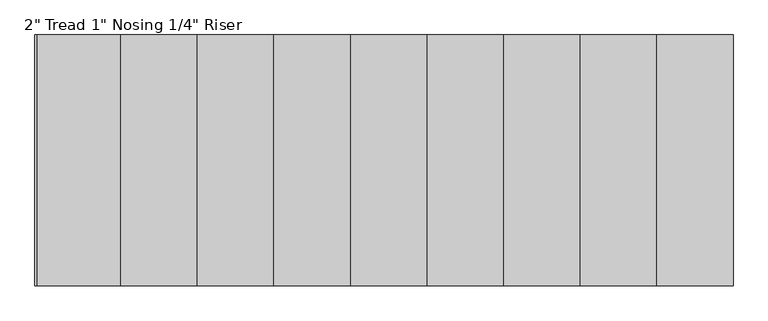
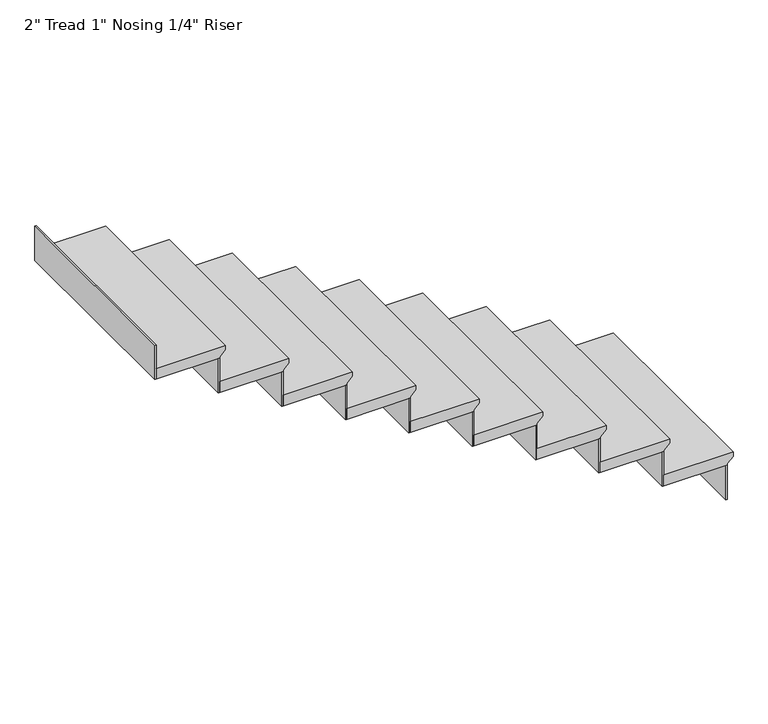
"""IFC4 building model written with IfcOpenShell, lengths in millimetres: stair flight geometry."""

from ifc_helpers import new_model, si_unit, frame, origin, place, context, project, spatial, polyline, outline, extrude, source, transform, mapped, element, save


def stair_flight_a571a0bd(model_context):
    return source(origin(), model_context, "Body", "SweptSolid", [
        extrude(outline(polyline([(8161.02, 923.4845537), (8161.02, 618.6845537), (8110.22, 618.6845537), (8110.22, 898.0845537), (8116.57, 898.0845537), (8141.97, 923.4845537), (8161.02, 923.4845537)])), frame((0.0, -5753.3544725, 0.0), z_axis=(0.0, 1.0, 0.0), x_axis=(0.0, 0.0, 1.0)), (0.0, 0.0, 1.0), 914.4),
        extrude(outline(polyline([(891.7345537, -4838.9544725), (898.0845537, -4838.9544725), (898.0845537, -5753.3544725), (891.7345537, -5753.3544725), (891.7345537, -4838.9544725)])), frame((0.0, 0.0, 7950.2), z_axis=(0.0, 0.0, 1.0), x_axis=(1.0, 0.0, 0.0)), (0.0, 0.0, 1.0), 160.02),
        extrude(outline(polyline([(612.3345537, -4838.9544725), (618.6845537, -4838.9544725), (618.6845537, -5753.3544725), (612.3345537, -5753.3544725), (612.3345537, -4838.9544725)])), frame((0.0, 0.0, 8110.22), z_axis=(0.0, 0.0, 1.0), x_axis=(1.0, 0.0, 0.0)), (0.0, 0.0, 1.0), 160.02),
        extrude(outline(polyline([(8321.04, 644.0845537), (8321.04, 339.2845537), (8270.24, 339.2845537), (8270.24, 618.6845537), (8276.59, 618.6845537), (8301.99, 644.0845537), (8321.04, 644.0845537)])), frame((0.0, -5753.3544725, 0.0), z_axis=(0.0, 1.0, 0.0), x_axis=(0.0, 0.0, 1.0)), (0.0, 0.0, 1.0), 914.4),
        extrude(outline(polyline([(332.9345537, -4838.9544725), (339.2845537, -4838.9544725), (339.2845537, -5753.3544725), (332.9345537, -5753.3544725), (332.9345537, -4838.9544725)])), frame((0.0, 0.0, 8270.24), z_axis=(0.0, 0.0, 1.0), x_axis=(1.0, 0.0, 0.0)), (0.0, 0.0, 1.0), 160.02),
        extrude(outline(polyline([(8481.06, 364.6845537), (8481.06, 59.8845537), (8430.26, 59.8845537), (8430.26, 339.2845537), (8436.61, 339.2845537), (8462.01, 364.6845537), (8481.06, 364.6845537)])), frame((0.0, -5753.3544725, 0.0), z_axis=(0.0, 1.0, 0.0), x_axis=(0.0, 0.0, 1.0)), (0.0, 0.0, 1.0), 914.4),
        extrude(outline(polyline([(53.5345537, -4838.9544725), (59.8845537, -4838.9544725), (59.8845537, -5753.3544725), (53.5345537, -5753.3544725), (53.5345537, -4838.9544725)])), frame((0.0, 0.0, 8430.26), z_axis=(0.0, 0.0, 1.0), x_axis=(1.0, 0.0, 0.0)), (0.0, 0.0, 1.0), 160.02),
        extrude(outline(polyline([(8641.08, 85.2845537), (8641.08, -219.5154463), (8590.28, -219.5154463), (8590.28, 59.8845537), (8596.63, 59.8845537), (8622.03, 85.2845537), (8641.08, 85.2845537)])), frame((0.0, -5753.3544725, 0.0), z_axis=(0.0, 1.0, 0.0), x_axis=(0.0, 0.0, 1.0)), (0.0, 0.0, 1.0), 914.4),
        extrude(outline(polyline([(-225.8654463, -4838.9544725), (-219.5154463, -4838.9544725), (-219.5154463, -5753.3544725), (-225.8654463, -5753.3544725), (-225.8654463, -4838.9544725)])), frame((0.0, 0.0, 8590.28), z_axis=(0.0, 0.0, 1.0), x_axis=(1.0, 0.0, 0.0)), (0.0, 0.0, 1.0), 160.02),
        extrude(outline(polyline([(8801.1, -194.1154463), (8801.1, -498.9154463), (8750.3, -498.9154463), (8750.3, -219.5154463), (8756.65, -219.5154463), (8782.05, -194.1154463), (8801.1, -194.1154463)])), frame((0.0, -5753.3544725, 0.0), z_axis=(0.0, 1.0, 0.0), x_axis=(0.0, 0.0, 1.0)), (0.0, 0.0, 1.0), 914.4),
        extrude(outline(polyline([(-505.2654463, -4838.9544725), (-498.9154463, -4838.9544725), (-498.9154463, -5753.3544725), (-505.2654463, -5753.3544725), (-505.2654463, -4838.9544725)])), frame((0.0, 0.0, 8750.3), z_axis=(0.0, 0.0, 1.0), x_axis=(1.0, 0.0, 0.0)), (0.0, 0.0, 1.0), 160.02),
        extrude(outline(polyline([(8961.12, -473.5154463), (8961.12, -778.3154463), (8910.32, -778.3154463), (8910.32, -498.9154463), (8916.67, -498.9154463), (8942.07, -473.5154463), (8961.12, -473.5154463)])), frame((0.0, -5753.3544725, 0.0), z_axis=(0.0, 1.0, 0.0), x_axis=(0.0, 0.0, 1.0)), (0.0, 0.0, 1.0), 914.4),
        extrude(outline(polyline([(-784.6654463, -4838.9544725), (-778.3154463, -4838.9544725), (-778.3154463, -5753.3544725), (-784.6654463, -5753.3544725), (-784.6654463, -4838.9544725)])), frame((0.0, 0.0, 8910.32), z_axis=(0.0, 0.0, 1.0), x_axis=(1.0, 0.0, 0.0)), (0.0, 0.0, 1.0), 160.02),
        extrude(outline(polyline([(9121.14, -752.9154463), (9121.14, -1057.7154463), (9070.34, -1057.7154463), (9070.34, -778.3154463), (9076.69, -778.3154463), (9102.09, -752.9154463), (9121.14, -752.9154463)])), frame((0.0, -5753.3544725, 0.0), z_axis=(0.0, 1.0, 0.0), x_axis=(0.0, 0.0, 1.0)), (0.0, 0.0, 1.0), 914.4),
        extrude(outline(polyline([(-1064.0654463, -4838.9544725), (-1057.7154463, -4838.9544725), (-1057.7154463, -5753.3544725), (-1064.0654463, -5753.3544725), (-1064.0654463, -4838.9544725)])), frame((0.0, 0.0, 9070.34), z_axis=(0.0, 0.0, 1.0), x_axis=(1.0, 0.0, 0.0)), (0.0, 0.0, 1.0), 160.02),
        extrude(outline(polyline([(9281.16, -1032.3154463), (9281.16, -1337.1154463), (9230.36, -1337.1154463), (9230.36, -1057.7154463), (9236.71, -1057.7154463), (9262.11, -1032.3154463), (9281.16, -1032.3154463)])), frame((0.0, -5753.3544725, 0.0), z_axis=(0.0, 1.0, 0.0), x_axis=(0.0, 0.0, 1.0)), (0.0, 0.0, 1.0), 914.4),
        extrude(outline(polyline([(-1343.4654463, -4838.9544725), (-1337.1154463, -4838.9544725), (-1337.1154463, -5753.3544725), (-1343.4654463, -5753.3544725), (-1343.4654463, -4838.9544725)])), frame((0.0, 0.0, 9230.36), z_axis=(0.0, 0.0, 1.0), x_axis=(1.0, 0.0, 0.0)), (0.0, 0.0, 1.0), 160.02),
        extrude(outline(polyline([(-1622.8654463, -4838.9544725), (-1616.5154463, -4838.9544725), (-1616.5154463, -5753.3544725), (-1622.8654463, -5753.3544725), (-1622.8654463, -4838.9544725)])), frame((0.0, 0.0, 9390.38), z_axis=(0.0, 0.0, 1.0), x_axis=(1.0, 0.0, 0.0)), (0.0, 0.0, 1.0), 160.02),
        extrude(outline(polyline([(9441.18, -1311.7154463), (9441.18, -1616.5154463), (9390.38, -1616.5154463), (9390.38, -1337.1154463), (9396.73, -1337.1154463), (9422.13, -1311.7154463), (9441.18, -1311.7154463)])), frame((0.0, -5753.3544725, 0.0), z_axis=(0.0, 1.0, 0.0), x_axis=(0.0, 0.0, 1.0)), (0.0, 0.0, 1.0), 914.4),
    ])


if __name__ == "__main__":
    model = new_model("IFC4")
    model_context = context("Model", 3, world=origin())
    ifc_project = project(units=[si_unit("LENGTHUNIT", "METRE", prefix="MILLI")], contexts=[model_context])
    site = spatial("IfcSite", under=ifc_project)
    building = spatial("IfcBuilding", under=site)
    placement = place(None, origin())
    stair_flight_shape = stair_flight_a571a0bd(model_context)
    element("IfcStairFlight", 1, ObjectType="2\" Tread 1\" Nosing 1/4\" Riser", at=placement, inside=building, context=model_context, shape_type="MappedRepresentation", body=[
        mapped(stair_flight_shape, transform((0.0, 0.0, 0.0), x_axis=(1.0, 0.0, 0.0), y_axis=(0.0, 1.0, 0.0), z_axis=(0.0, 0.0, 1.0))),
    ])
    save(model, "model.ifc")
